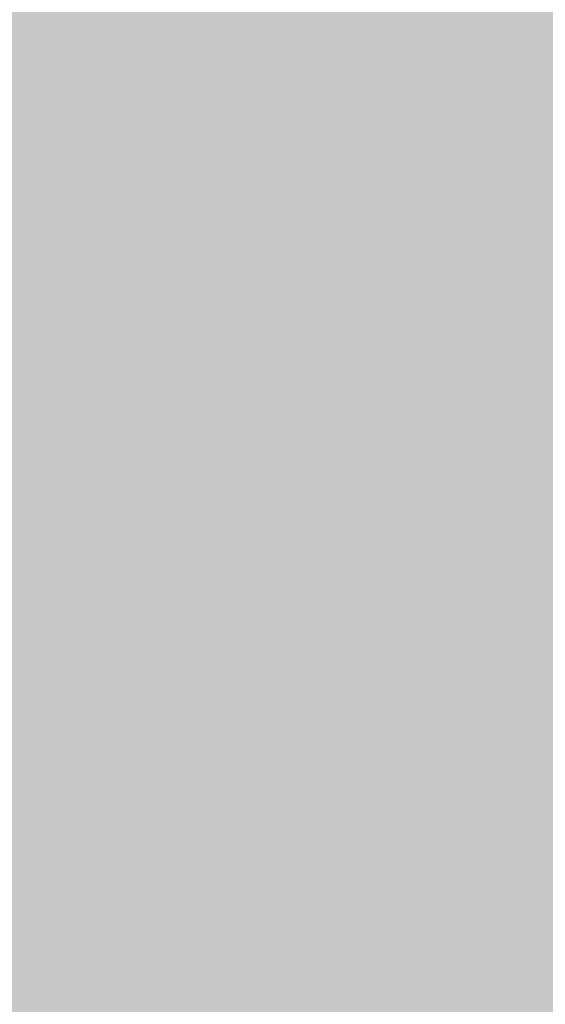
# Model space of a CAD drawing. Units: millimetres. Extents: x -22994 to 29398, y -19990 to 20176.
# Tile 61 of 135: x 225.441 to 227.437, y 79.586 to 83.328. Entities that reach past the tile are written whole.
import ezdxf
from ezdxf import colors
from ezdxf.entities.mleader import LeaderData, LeaderLine
from ezdxf.math import Vec2, Vec3

# ---------------------------------------------------------------- set-up
doc = ezdxf.new("R2010")
doc.units = ezdxf.units.MM
doc.header["$MEASUREMENT"] = 0
doc.layers.add('M-ANNO-TEXT', color=7, linetype='Continuous', lineweight=25)
doc.layers.add('M-DIMS', color=2, linetype='Continuous', lineweight=18)
doc.styles.get("Standard").update_dxf_attribs({"font": 'arial.ttf'})
doc.dimstyles.get("Standard").update_dxf_attribs({"dimtxt": 0.18, "dimasz": 10000, "dimexe": 0.18, "dimexo": 0.0625, "dimgap": 0.09, "dimtad": 0, "dimtih": 1, "dimtoh": 1, "dimdec": 0, "dimzin": 0, "dimdsep": 46, "dimtxsty": 'Standard', "dimcen": 0.09, "dimadec": 0, "dimazin": 0, "dimtfac": 1, "dimtdec": 0, "dimtofl": 0, "dimtmove": 0, "dimatfit": 3, "dimfxl": 1, "dimtolj": 1, "dimtzin": 0, "dimlwd": 30, "dimarcsym": 0})

# ---------------------------------------------------------------- blocks, each defined once
blk = doc.blocks.new('*D2')
at = {"layer": 'Defpoints', "color": 0, "transparency": 16777216}
for p in [(6.6773, 10.2713), (290.852, 10.2713), (290.852, -5.0787)]:
    blk.add_point(p, dxfattribs=at)
at = {"layer": 'M-DIMS', "color": 0, "lineweight": -2, "transparency": 16777216}
for p, q in [((6.6773, 10.2088), (6.6773, -5.2587)), ((290.852, 10.2088), (290.852, -5.2587))]:
    blk.add_line(p, q, dxfattribs=at)
at = {"layer": 'M-DIMS', "color": 0, "lineweight": 30, "transparency": 16777216}
for p, q in [((-9993.3227, -5.0787), (-19993.3227, -5.0787)), ((10290.852, -5.0787), (20290.852, -5.0787))]:
    blk.add_line(p, q, dxfattribs=at)
at = {"layer": 'M-DIMS', "color": 0, "transparency": 16777216}
for points in [[(-9993.3227, 1661.5879), (-9993.3227, -1671.7454), (6.6773, -5.0787)], [(10290.852, 1661.5879), (10290.852, -1671.7454), (290.852, -5.0787)]]:
    blk.add_solid(points, dxfattribs=at)
at = {"layer": 'M-DIMS', "color": 0, "transparency": 16777216, "insert": (148.7647, -5.0787), "char_height": 0.18, "attachment_point": 5}
blk.add_mtext('\\A1;284.2', dxfattribs=at)
blk = doc.blocks.new('*D3')
at = {"layer": 'Defpoints', "color": 0, "transparency": 16777216}
for p in [(110.2647, 204.1654), (110.2647, 176.3662), (95.8327, 127.967)]:
    blk.add_point(p, dxfattribs=at)
at = {"layer": 'M-DIMS', "color": 0, "lineweight": -2, "transparency": 16777216}
for p, q in [((95.8327, 128.0295), (95.8327, 204.3454)), ((110.2647, 176.4287), (110.2647, 204.3454))]:
    blk.add_line(p, q, dxfattribs=at)
at = {"layer": 'M-DIMS', "color": 0, "lineweight": 30, "transparency": 16777216}
for p, q in [((-9904.1673, 204.1654), (-19904.1673, 204.1654)), ((10110.2647, 204.1654), (20110.2647, 204.1654))]:
    blk.add_line(p, q, dxfattribs=at)
at = {"layer": 'M-DIMS', "color": 0, "transparency": 16777216}
for points in [[(-9904.1673, 1870.8321), (-9904.1673, -1462.5013), (95.8327, 204.1654)], [(10110.2647, 1870.8321), (10110.2647, -1462.5013), (110.2647, 204.1654)]]:
    blk.add_solid(points, dxfattribs=at)
at = {"layer": 'M-DIMS', "color": 0, "transparency": 16777216, "insert": (103.0487, 204.1654), "char_height": 0.18, "attachment_point": 5}
blk.add_mtext('\\A1;14.432', dxfattribs=at)
blk = doc.blocks.new('*D4')
at = {"layer": 'Defpoints', "color": 0, "transparency": 16777216}
for p in [(116.2647, 204.1654), (110.2647, 176.3662), (116.2647, 176.3662)]:
    blk.add_point(p, dxfattribs=at)
at = {"layer": 'M-DIMS', "color": 0, "lineweight": -2, "transparency": 16777216}
for p, q in [((110.2647, 176.4287), (110.2647, 204.3454)), ((116.2647, 176.4287), (116.2647, 204.3454))]:
    blk.add_line(p, q, dxfattribs=at)
at = {"layer": 'M-DIMS', "color": 0, "lineweight": 30, "transparency": 16777216}
for p, q in [((-9889.7353, 204.1654), (-19889.7353, 204.1654)), ((10116.2647, 204.1654), (20116.2647, 204.1654))]:
    blk.add_line(p, q, dxfattribs=at)
at = {"layer": 'M-DIMS', "color": 0, "transparency": 16777216}
for points in [[(-9889.7353, 1870.8321), (-9889.7353, -1462.5013), (110.2647, 204.1654)], [(10116.2647, 1870.8321), (10116.2647, -1462.5013), (116.2647, 204.1654)]]:
    blk.add_solid(points, dxfattribs=at)
at = {"layer": 'M-DIMS', "color": 0, "transparency": 16777216, "insert": (113.2647, 204.1654), "char_height": 0.18, "attachment_point": 5}
blk.add_mtext('\\A1;6', dxfattribs=at)
blk = doc.blocks.new('*D5')
at = {"layer": 'Defpoints', "color": 0, "transparency": 16777216}
for p in [(181.2647, 204.1654), (116.2647, 176.3662), (181.2647, 176.3662)]:
    blk.add_point(p, dxfattribs=at)
at = {"layer": 'M-DIMS', "color": 0, "lineweight": -2, "transparency": 16777216}
for p, q in [((116.2647, 176.4287), (116.2647, 204.3454)), ((181.2647, 176.4287), (181.2647, 204.3454))]:
    blk.add_line(p, q, dxfattribs=at)
at = {"layer": 'M-DIMS', "color": 0, "lineweight": 30, "transparency": 16777216}
for p, q in [((-9883.7353, 204.1654), (-19883.7353, 204.1654)), ((10181.2647, 204.1654), (20181.2647, 204.1654))]:
    blk.add_line(p, q, dxfattribs=at)
at = {"layer": 'M-DIMS', "color": 0, "transparency": 16777216}
for points in [[(-9883.7353, 1870.8321), (-9883.7353, -1462.5013), (116.2647, 204.1654)], [(10181.2647, 1870.8321), (10181.2647, -1462.5013), (181.2647, 204.1654)]]:
    blk.add_solid(points, dxfattribs=at)
at = {"layer": 'M-DIMS', "color": 0, "transparency": 16777216, "insert": (148.7647, 204.1654), "char_height": 0.18, "attachment_point": 5}
blk.add_mtext('\\A1;65', dxfattribs=at)
blk = doc.blocks.new('*D6')
at = {"layer": 'Defpoints', "color": 0, "transparency": 16777216}
for p in [(187.2647, 204.1654), (181.2647, 176.3662), (187.2647, 176.3662)]:
    blk.add_point(p, dxfattribs=at)
at = {"layer": 'M-DIMS', "color": 0, "lineweight": -2, "transparency": 16777216}
for p, q in [((181.2647, 176.4287), (181.2647, 204.3454)), ((187.2647, 176.4287), (187.2647, 204.3454))]:
    blk.add_line(p, q, dxfattribs=at)
at = {"layer": 'M-DIMS', "color": 0, "lineweight": 30, "transparency": 16777216}
for p, q in [((-9818.7353, 204.1654), (-19818.7353, 204.1654)), ((10187.2647, 204.1654), (20187.2647, 204.1654))]:
    blk.add_line(p, q, dxfattribs=at)
at = {"layer": 'M-DIMS', "color": 0, "transparency": 16777216}
for points in [[(-9818.7353, 1870.8321), (-9818.7353, -1462.5013), (181.2647, 204.1654)], [(10187.2647, 1870.8321), (10187.2647, -1462.5013), (187.2647, 204.1654)]]:
    blk.add_solid(points, dxfattribs=at)
at = {"layer": 'M-DIMS', "color": 0, "transparency": 16777216, "insert": (184.2647, 204.1654), "char_height": 0.18, "attachment_point": 5}
blk.add_mtext('\\A1;6', dxfattribs=at)
blk = doc.blocks.new('*D7')
at = {"layer": 'Defpoints', "color": 0, "transparency": 16777216}
for p in [(201.6967, 204.1654), (187.2647, 176.3662), (201.6967, 127.967)]:
    blk.add_point(p, dxfattribs=at)
at = {"layer": 'M-DIMS', "color": 0, "lineweight": -2, "transparency": 16777216}
for p, q in [((187.2647, 176.4287), (187.2647, 204.3454)), ((201.6967, 128.0295), (201.6967, 204.3454))]:
    blk.add_line(p, q, dxfattribs=at)
at = {"layer": 'M-DIMS', "color": 0, "lineweight": 30, "transparency": 16777216}
for p, q in [((-9812.7353, 204.1654), (-19812.7353, 204.1654)), ((10201.6967, 204.1654), (20201.6967, 204.1654))]:
    blk.add_line(p, q, dxfattribs=at)
at = {"layer": 'M-DIMS', "color": 0, "transparency": 16777216}
for points in [[(-9812.7353, 1870.8321), (-9812.7353, -1462.5013), (187.2647, 204.1654)], [(10201.6967, 1870.8321), (10201.6967, -1462.5013), (201.6967, 204.1654)]]:
    blk.add_solid(points, dxfattribs=at)
at = {"layer": 'M-DIMS', "color": 0, "transparency": 16777216, "insert": (194.4807, 204.1654), "char_height": 0.18, "attachment_point": 5}
blk.add_mtext('\\A1;14.432', dxfattribs=at)
blk = doc.blocks.new('*D8')
at = {"layer": 'Defpoints', "color": 0, "transparency": 16777216}
for p in [(227.6485, 204.1654), (227.6485, 146.7296), (201.6967, 127.967)]:
    blk.add_point(p, dxfattribs=at)
at = {"layer": 'M-DIMS', "color": 0, "lineweight": -2, "transparency": 16777216}
for p, q in [((201.6967, 128.0295), (201.6967, 204.3454)), ((227.6485, 146.7921), (227.6485, 204.3454))]:
    blk.add_line(p, q, dxfattribs=at)
at = {"layer": 'M-DIMS', "color": 0, "lineweight": 30, "transparency": 16777216}
for p, q in [((-9798.3033, 204.1654), (-19798.3033, 204.1654)), ((10227.6485, 204.1654), (20227.6485, 204.1654))]:
    blk.add_line(p, q, dxfattribs=at)
at = {"layer": 'M-DIMS', "color": 0, "transparency": 16777216}
for points in [[(-9798.3033, 1870.8321), (-9798.3033, -1462.5013), (201.6967, 204.1654)], [(10227.6485, 1870.8321), (10227.6485, -1462.5013), (227.6485, 204.1654)]]:
    blk.add_solid(points, dxfattribs=at)
at = {"layer": 'M-DIMS', "color": 0, "transparency": 16777216, "insert": (214.6726, 204.1654), "char_height": 0.18, "attachment_point": 5}
blk.add_mtext('\\A1;25.95', dxfattribs=at)
blk = doc.blocks.new('*D9')
at = {"layer": 'Defpoints', "color": 0, "transparency": 16777216}
for p in [(187.2647, 176.3662), (306.202, 176.3662), (290.852, 10.2713)]:
    blk.add_point(p, dxfattribs=at)
at = {"layer": 'M-DIMS', "color": 0, "lineweight": 30, "transparency": 16777216}
for p, q in [((306.202, 10176.3662), (306.202, 20176.3662)), ((306.202, -9989.7287), (306.202, -19989.7287))]:
    blk.add_line(p, q, dxfattribs=at)
at = {"layer": 'M-DIMS', "color": 0, "lineweight": -2, "transparency": 16777216}
for p, q in [((187.3272, 176.3662), (306.382, 176.3662)), ((290.9145, 10.2713), (306.382, 10.2713))]:
    blk.add_line(p, q, dxfattribs=at)
at = {"layer": 'M-DIMS', "color": 0, "transparency": 16777216}
for points in [[(-1360.4646, 10176.3662), (1972.8687, 10176.3662), (306.202, 176.3662)], [(-1360.4646, -9989.7287), (1972.8687, -9989.7287), (306.202, 10.2713)]]:
    blk.add_solid(points, dxfattribs=at)
at = {"layer": 'M-DIMS', "color": 0, "transparency": 16777216, "insert": (306.202, 93.3187), "char_height": 0.18, "attachment_point": 5}
blk.add_mtext('\\A1;166.1', dxfattribs=at)
blk = doc.blocks.new('*D10')
at = {"layer": 'Defpoints', "color": 0, "transparency": 16777216}
for p in [(125.6498, 136.0713), (133.3459, 136.0713), (133.3459, -5.0787)]:
    blk.add_point(p, dxfattribs=at)
at = {"layer": 'M-DIMS', "color": 0, "lineweight": -2, "transparency": 16777216}
for p, q in [((125.6498, 136.0088), (125.6498, -5.2587)), ((133.3459, 136.0088), (133.3459, -5.2587))]:
    blk.add_line(p, q, dxfattribs=at)
at = {"layer": 'M-DIMS', "color": 0, "lineweight": 30, "transparency": 16777216}
for p, q in [((-9874.3502, -5.0787), (-19874.3502, -5.0787)), ((10133.3459, -5.0787), (20133.3459, -5.0787))]:
    blk.add_line(p, q, dxfattribs=at)
at = {"layer": 'M-DIMS', "color": 0, "transparency": 16777216}
for points in [[(-9874.3502, 1661.5879), (-9874.3502, -1671.7454), (125.6498, -5.0787)], [(10133.3459, 1661.5879), (10133.3459, -1671.7454), (133.3459, -5.0787)]]:
    blk.add_solid(points, dxfattribs=at)
at = {"layer": 'M-DIMS', "color": 0, "transparency": 16777216, "insert": (129.4978, -5.0787), "char_height": 0.18, "attachment_point": 5}
blk.add_mtext('\\A1;7.696', dxfattribs=at)
blk = doc.blocks.new('*D11')
at = {"layer": 'Defpoints', "color": 0, "transparency": 16777216}
for p in [(133.3459, 136.0713), (135.6498, 136.0713), (135.6498, -5.0787)]:
    blk.add_point(p, dxfattribs=at)
at = {"layer": 'M-DIMS', "color": 0, "lineweight": -2, "transparency": 16777216}
for p, q in [((133.3459, 136.0088), (133.3459, -5.2587)), ((135.6498, 136.0088), (135.6498, -5.2587))]:
    blk.add_line(p, q, dxfattribs=at)
at = {"layer": 'M-DIMS', "color": 0, "lineweight": 30, "transparency": 16777216}
for p, q in [((-9866.6541, -5.0787), (-19866.6541, -5.0787)), ((10135.6498, -5.0787), (20135.6498, -5.0787))]:
    blk.add_line(p, q, dxfattribs=at)
at = {"layer": 'M-DIMS', "color": 0, "transparency": 16777216}
for points in [[(-9866.6541, 1661.5879), (-9866.6541, -1671.7454), (133.3459, -5.0787)], [(10135.6498, 1661.5879), (10135.6498, -1671.7454), (135.6498, -5.0787)]]:
    blk.add_solid(points, dxfattribs=at)
at = {"layer": 'M-DIMS', "color": 0, "transparency": 16777216, "insert": (134.4978, -5.0787), "char_height": 0.18, "attachment_point": 5}
blk.add_mtext('\\A1;2.304', dxfattribs=at)
blk = doc.blocks.new('*D12')
at = {"layer": 'Defpoints', "color": 0, "transparency": 16777216}
for p in [(135.6498, 136.0713), (145.6498, 136.0713), (145.6498, -5.0787)]:
    blk.add_point(p, dxfattribs=at)
at = {"layer": 'M-DIMS', "color": 0, "lineweight": -2, "transparency": 16777216}
for p, q in [((135.6498, 136.0088), (135.6498, -5.2587)), ((145.6498, 136.0088), (145.6498, -5.2587))]:
    blk.add_line(p, q, dxfattribs=at)
at = {"layer": 'M-DIMS', "color": 0, "lineweight": 30, "transparency": 16777216}
for p, q in [((-9864.3502, -5.0787), (-19864.3502, -5.0787)), ((10145.6498, -5.0787), (20145.6498, -5.0787))]:
    blk.add_line(p, q, dxfattribs=at)
at = {"layer": 'M-DIMS', "color": 0, "transparency": 16777216}
for points in [[(-9864.3502, 1661.5879), (-9864.3502, -1671.7454), (135.6498, -5.0787)], [(10145.6498, 1661.5879), (10145.6498, -1671.7454), (145.6498, -5.0787)]]:
    blk.add_solid(points, dxfattribs=at)
at = {"layer": 'M-DIMS', "color": 0, "transparency": 16777216, "insert": (140.6498, -5.0787), "char_height": 0.18, "attachment_point": 5}
blk.add_mtext('\\A1;10', dxfattribs=at)
blk = doc.blocks.new('*D13')
at = {"layer": 'Defpoints', "color": 0, "transparency": 16777216}
for p in [(145.6498, 136.0713), (155.6498, 136.0713), (155.6498, -5.0787)]:
    blk.add_point(p, dxfattribs=at)
at = {"layer": 'M-DIMS', "color": 0, "lineweight": -2, "transparency": 16777216}
for p, q in [((145.6498, 136.0088), (145.6498, -5.2587)), ((155.6498, 136.0088), (155.6498, -5.2587))]:
    blk.add_line(p, q, dxfattribs=at)
at = {"layer": 'M-DIMS', "color": 0, "lineweight": 30, "transparency": 16777216}
for p, q in [((-9854.3502, -5.0787), (-19854.3502, -5.0787)), ((10155.6498, -5.0787), (20155.6498, -5.0787))]:
    blk.add_line(p, q, dxfattribs=at)
at = {"layer": 'M-DIMS', "color": 0, "transparency": 16777216}
for points in [[(-9854.3502, 1661.5879), (-9854.3502, -1671.7454), (145.6498, -5.0787)], [(10155.6498, 1661.5879), (10155.6498, -1671.7454), (155.6498, -5.0787)]]:
    blk.add_solid(points, dxfattribs=at)
at = {"layer": 'M-DIMS', "color": 0, "transparency": 16777216, "insert": (150.6498, -5.0787), "char_height": 0.18, "attachment_point": 5}
blk.add_mtext('\\A1;10', dxfattribs=at)
blk = doc.blocks.new('*D14')
at = {"layer": 'Defpoints', "color": 0, "transparency": 16777216}
for p in [(155.6498, 136.0713), (165.6498, 136.0713), (165.6498, -5.0787)]:
    blk.add_point(p, dxfattribs=at)
at = {"layer": 'M-DIMS', "color": 0, "lineweight": -2, "transparency": 16777216}
for p, q in [((155.6498, 136.0088), (155.6498, -5.2587)), ((165.6498, 136.0088), (165.6498, -5.2587))]:
    blk.add_line(p, q, dxfattribs=at)
at = {"layer": 'M-DIMS', "color": 0, "lineweight": 30, "transparency": 16777216}
for p, q in [((-9844.3502, -5.0787), (-19844.3502, -5.0787)), ((10165.6498, -5.0787), (20165.6498, -5.0787))]:
    blk.add_line(p, q, dxfattribs=at)
at = {"layer": 'M-DIMS', "color": 0, "transparency": 16777216}
for points in [[(-9844.3502, 1661.5879), (-9844.3502, -1671.7454), (155.6498, -5.0787)], [(10165.6498, 1661.5879), (10165.6498, -1671.7454), (165.6498, -5.0787)]]:
    blk.add_solid(points, dxfattribs=at)
at = {"layer": 'M-DIMS', "color": 0, "transparency": 16777216, "insert": (160.6498, -5.0787), "char_height": 0.18, "attachment_point": 5}
blk.add_mtext('\\A1;10', dxfattribs=at)
blk = doc.blocks.new('*D15')
at = {"layer": 'Defpoints', "color": 0, "transparency": 16777216}
for p in [(173.3459, 154.788), (173.3459, 136.0713), (306.202, 136.0713)]:
    blk.add_point(p, dxfattribs=at)
at = {"layer": 'M-DIMS', "color": 0, "lineweight": 30, "transparency": 16777216}
for p, q in [((306.202, 10154.788), (306.202, 20154.788)), ((306.202, -9863.9287), (306.202, -19863.9287))]:
    blk.add_line(p, q, dxfattribs=at)
at = {"layer": 'M-DIMS', "color": 0, "lineweight": -2, "transparency": 16777216}
for p, q in [((173.4084, 154.788), (306.382, 154.788)), ((173.4084, 136.0713), (306.382, 136.0713))]:
    blk.add_line(p, q, dxfattribs=at)
at = {"layer": 'M-DIMS', "color": 0, "transparency": 16777216}
for points in [[(-1360.4646, 10154.788), (1972.8687, 10154.788), (306.202, 154.788)], [(-1360.4646, -9863.9287), (1972.8687, -9863.9287), (306.202, 136.0713)]]:
    blk.add_solid(points, dxfattribs=at)
at = {"layer": 'M-DIMS', "color": 0, "transparency": 16777216, "insert": (306.202, 145.4297), "char_height": 0.18, "attachment_point": 5}
blk.add_mtext('\\A1;18.717', dxfattribs=at)
blk = doc.blocks.new('*D16')
at = {"layer": 'Defpoints', "color": 0, "transparency": 16777216}
for p in [(120.1702, 204.1654), (110.4658, 48.0349), (120.1702, 48.0349)]:
    blk.add_point(p, dxfattribs=at)
at = {"layer": 'M-DIMS', "color": 0, "lineweight": -2, "transparency": 16777216}
for p, q in [((110.4658, 48.0974), (110.4658, 204.3454)), ((120.1702, 48.0974), (120.1702, 204.3454))]:
    blk.add_line(p, q, dxfattribs=at)
at = {"layer": 'M-DIMS', "color": 0, "lineweight": 30, "transparency": 16777216}
for p, q in [((-9889.5342, 204.1654), (-19889.5342, 204.1654)), ((10120.1702, 204.1654), (20120.1702, 204.1654))]:
    blk.add_line(p, q, dxfattribs=at)
at = {"layer": 'M-DIMS', "color": 0, "transparency": 16777216}
for points in [[(-9889.5342, 1870.8321), (-9889.5342, -1462.5013), (110.4658, 204.1654)], [(10120.1702, 1870.8321), (10120.1702, -1462.5013), (120.1702, 204.1654)]]:
    blk.add_solid(points, dxfattribs=at)
at = {"layer": 'M-DIMS', "color": 0, "transparency": 16777216, "insert": (115.318, 204.1654), "char_height": 0.18, "attachment_point": 5}
blk.add_mtext('\\A1;9.704', dxfattribs=at)
blk = doc.blocks.new('*D17')
at = {"layer": 'Defpoints', "color": 0, "transparency": 16777216}
for p in [(126.1702, 204.1654), (120.1702, 48.0349), (126.1702, 48.0349)]:
    blk.add_point(p, dxfattribs=at)
at = {"layer": 'M-DIMS', "color": 0, "lineweight": -2, "transparency": 16777216}
for p, q in [((120.1702, 48.0974), (120.1702, 204.3454)), ((126.1702, 48.0974), (126.1702, 204.3454))]:
    blk.add_line(p, q, dxfattribs=at)
at = {"layer": 'M-DIMS', "color": 0, "lineweight": 30, "transparency": 16777216}
for p, q in [((-9879.8298, 204.1654), (-19879.8298, 204.1654)), ((10126.1702, 204.1654), (20126.1702, 204.1654))]:
    blk.add_line(p, q, dxfattribs=at)
at = {"layer": 'M-DIMS', "color": 0, "transparency": 16777216}
for points in [[(-9879.8298, 1870.8321), (-9879.8298, -1462.5013), (120.1702, 204.1654)], [(10126.1702, 1870.8321), (10126.1702, -1462.5013), (126.1702, 204.1654)]]:
    blk.add_solid(points, dxfattribs=at)
at = {"layer": 'M-DIMS', "color": 0, "transparency": 16777216, "insert": (123.1702, 204.1654), "char_height": 0.18, "attachment_point": 5}
blk.add_mtext('\\A1;6', dxfattribs=at)
blk = doc.blocks.new('*D18')
at = {"layer": 'Defpoints', "color": 0, "transparency": 16777216}
for p in [(132.1702, 204.1654), (126.1702, 48.0349), (132.1702, 48.0349)]:
    blk.add_point(p, dxfattribs=at)
at = {"layer": 'M-DIMS', "color": 0, "lineweight": -2, "transparency": 16777216}
for p, q in [((126.1702, 48.0974), (126.1702, 204.3454)), ((132.1702, 48.0974), (132.1702, 204.3454))]:
    blk.add_line(p, q, dxfattribs=at)
at = {"layer": 'M-DIMS', "color": 0, "lineweight": 30, "transparency": 16777216}
for p, q in [((-9873.8298, 204.1654), (-19873.8298, 204.1654)), ((10132.1702, 204.1654), (20132.1702, 204.1654))]:
    blk.add_line(p, q, dxfattribs=at)
at = {"layer": 'M-DIMS', "color": 0, "transparency": 16777216}
for points in [[(-9873.8298, 1870.8321), (-9873.8298, -1462.5013), (126.1702, 204.1654)], [(10132.1702, 1870.8321), (10132.1702, -1462.5013), (132.1702, 204.1654)]]:
    blk.add_solid(points, dxfattribs=at)
at = {"layer": 'M-DIMS', "color": 0, "transparency": 16777216, "insert": (129.1702, 204.1654), "char_height": 0.18, "attachment_point": 5}
blk.add_mtext('\\A1;6', dxfattribs=at)
blk = doc.blocks.new('*D19')
at = {"layer": 'Defpoints', "color": 0, "transparency": 16777216}
for p in [(138.1702, 204.1654), (132.1702, 48.0349), (138.1702, 48.0349)]:
    blk.add_point(p, dxfattribs=at)
at = {"layer": 'M-DIMS', "color": 0, "lineweight": -2, "transparency": 16777216}
for p, q in [((132.1702, 48.0974), (132.1702, 204.3454)), ((138.1702, 48.0974), (138.1702, 204.3454))]:
    blk.add_line(p, q, dxfattribs=at)
at = {"layer": 'M-DIMS', "color": 0, "lineweight": 30, "transparency": 16777216}
for p, q in [((-9867.8298, 204.1654), (-19867.8298, 204.1654)), ((10138.1702, 204.1654), (20138.1702, 204.1654))]:
    blk.add_line(p, q, dxfattribs=at)
at = {"layer": 'M-DIMS', "color": 0, "transparency": 16777216}
for points in [[(-9867.8298, 1870.8321), (-9867.8298, -1462.5013), (132.1702, 204.1654)], [(10138.1702, 1870.8321), (10138.1702, -1462.5013), (138.1702, 204.1654)]]:
    blk.add_solid(points, dxfattribs=at)
at = {"layer": 'M-DIMS', "color": 0, "transparency": 16777216, "insert": (135.1702, 204.1654), "char_height": 0.18, "attachment_point": 5}
blk.add_mtext('\\A1;6', dxfattribs=at)
blk = doc.blocks.new('*D20')
at = {"layer": 'Defpoints', "color": 0, "transparency": 16777216}
for p in [(144.1702, 204.1654), (138.1702, 48.0349), (144.1702, 48.0349)]:
    blk.add_point(p, dxfattribs=at)
at = {"layer": 'M-DIMS', "color": 0, "lineweight": -2, "transparency": 16777216}
for p, q in [((138.1702, 48.0974), (138.1702, 204.3454)), ((144.1702, 48.0974), (144.1702, 204.3454))]:
    blk.add_line(p, q, dxfattribs=at)
at = {"layer": 'M-DIMS', "color": 0, "lineweight": 30, "transparency": 16777216}
for p, q in [((-9861.8298, 204.1654), (-19861.8298, 204.1654)), ((10144.1702, 204.1654), (20144.1702, 204.1654))]:
    blk.add_line(p, q, dxfattribs=at)
at = {"layer": 'M-DIMS', "color": 0, "transparency": 16777216}
for points in [[(-9861.8298, 1870.8321), (-9861.8298, -1462.5013), (138.1702, 204.1654)], [(10144.1702, 1870.8321), (10144.1702, -1462.5013), (144.1702, 204.1654)]]:
    blk.add_solid(points, dxfattribs=at)
at = {"layer": 'M-DIMS', "color": 0, "transparency": 16777216, "insert": (141.1702, 204.1654), "char_height": 0.18, "attachment_point": 5}
blk.add_mtext('\\A1;6', dxfattribs=at)
blk = doc.blocks.new('*D21')
at = {"layer": 'Defpoints', "color": 0, "transparency": 16777216}
for p in [(149.1157, 204.1654), (144.1702, 48.0349), (149.1157, 48.0349)]:
    blk.add_point(p, dxfattribs=at)
at = {"layer": 'M-DIMS', "color": 0, "lineweight": -2, "transparency": 16777216}
for p, q in [((144.1702, 48.0974), (144.1702, 204.3454)), ((149.1157, 48.0974), (149.1157, 204.3454))]:
    blk.add_line(p, q, dxfattribs=at)
at = {"layer": 'M-DIMS', "color": 0, "lineweight": 30, "transparency": 16777216}
for p, q in [((-9855.8298, 204.1654), (-19855.8298, 204.1654)), ((10149.1157, 204.1654), (20149.1157, 204.1654))]:
    blk.add_line(p, q, dxfattribs=at)
at = {"layer": 'M-DIMS', "color": 0, "transparency": 16777216}
for points in [[(-9855.8298, 1870.8321), (-9855.8298, -1462.5013), (144.1702, 204.1654)], [(10149.1157, 1870.8321), (10149.1157, -1462.5013), (149.1157, 204.1654)]]:
    blk.add_solid(points, dxfattribs=at)
at = {"layer": 'M-DIMS', "color": 0, "transparency": 16777216, "insert": (146.6429, 204.1654), "char_height": 0.18, "attachment_point": 5}
blk.add_mtext('\\A1;4.945', dxfattribs=at)
blk = doc.blocks.new('*D22')
at = {"layer": 'Defpoints', "color": 0, "transparency": 16777216}
for p in [(149.1157, 30.9895), (155.1157, 30.9895), (155.1157, -5.0787)]:
    blk.add_point(p, dxfattribs=at)
at = {"layer": 'M-DIMS', "color": 0, "lineweight": -2, "transparency": 16777216}
for p, q in [((149.1157, 30.927), (149.1157, -5.2587)), ((155.1157, 30.927), (155.1157, -5.2587))]:
    blk.add_line(p, q, dxfattribs=at)
at = {"layer": 'M-DIMS', "color": 0, "lineweight": 30, "transparency": 16777216}
for p, q in [((-9850.8843, -5.0787), (-19850.8843, -5.0787)), ((10155.1157, -5.0787), (20155.1157, -5.0787))]:
    blk.add_line(p, q, dxfattribs=at)
at = {"layer": 'M-DIMS', "color": 0, "transparency": 16777216}
for points in [[(-9850.8843, 1661.5879), (-9850.8843, -1671.7454), (149.1157, -5.0787)], [(10155.1157, 1661.5879), (10155.1157, -1671.7454), (155.1157, -5.0787)]]:
    blk.add_solid(points, dxfattribs=at)
at = {"layer": 'M-DIMS', "color": 0, "transparency": 16777216, "insert": (152.1157, -5.0787), "char_height": 0.18, "attachment_point": 5}
blk.add_mtext('\\A1;6', dxfattribs=at)
blk = doc.blocks.new('*D23')
at = {"layer": 'Defpoints', "color": 0, "transparency": 16777216}
for p in [(155.1157, 30.9895), (161.1157, 30.9895), (161.1157, -5.0787)]:
    blk.add_point(p, dxfattribs=at)
at = {"layer": 'M-DIMS', "color": 0, "lineweight": -2, "transparency": 16777216}
for p, q in [((155.1157, 30.927), (155.1157, -5.2587)), ((161.1157, 30.927), (161.1157, -5.2587))]:
    blk.add_line(p, q, dxfattribs=at)
at = {"layer": 'M-DIMS', "color": 0, "lineweight": 30, "transparency": 16777216}
for p, q in [((-9844.8843, -5.0787), (-19844.8843, -5.0787)), ((10161.1157, -5.0787), (20161.1157, -5.0787))]:
    blk.add_line(p, q, dxfattribs=at)
at = {"layer": 'M-DIMS', "color": 0, "transparency": 16777216}
for points in [[(-9844.8843, 1661.5879), (-9844.8843, -1671.7454), (155.1157, -5.0787)], [(10161.1157, 1661.5879), (10161.1157, -1671.7454), (161.1157, -5.0787)]]:
    blk.add_solid(points, dxfattribs=at)
at = {"layer": 'M-DIMS', "color": 0, "transparency": 16777216, "insert": (158.1157, -5.0787), "char_height": 0.18, "attachment_point": 5}
blk.add_mtext('\\A1;6', dxfattribs=at)
blk = doc.blocks.new('*D24')
at = {"layer": 'Defpoints', "color": 0, "transparency": 16777216}
for p in [(161.1157, 30.9895), (166.4387, 30.9895), (166.4387, -5.0787)]:
    blk.add_point(p, dxfattribs=at)
at = {"layer": 'M-DIMS', "color": 0, "lineweight": -2, "transparency": 16777216}
for p, q in [((161.1157, 30.927), (161.1157, -5.2587)), ((166.4387, 30.927), (166.4387, -5.2587))]:
    blk.add_line(p, q, dxfattribs=at)
at = {"layer": 'M-DIMS', "color": 0, "lineweight": 30, "transparency": 16777216}
for p, q in [((-9838.8843, -5.0787), (-19838.8843, -5.0787)), ((10166.4387, -5.0787), (20166.4387, -5.0787))]:
    blk.add_line(p, q, dxfattribs=at)
at = {"layer": 'M-DIMS', "color": 0, "transparency": 16777216}
for points in [[(-9838.8843, 1661.5879), (-9838.8843, -1671.7454), (161.1157, -5.0787)], [(10166.4387, 1661.5879), (10166.4387, -1671.7454), (166.4387, -5.0787)]]:
    blk.add_solid(points, dxfattribs=at)
at = {"layer": 'M-DIMS', "color": 0, "transparency": 16777216, "insert": (163.7772, -5.0787), "char_height": 0.18, "attachment_point": 5}
blk.add_mtext('\\A1;5.323', dxfattribs=at)
blk = doc.blocks.new('*D25')
at = {"layer": 'Defpoints', "color": 0, "transparency": 16777216}
for p in [(166.4387, 30.9895), (172.4387, 30.9895), (172.4387, -5.0787)]:
    blk.add_point(p, dxfattribs=at)
at = {"layer": 'M-DIMS', "color": 0, "lineweight": -2, "transparency": 16777216}
for p, q in [((166.4387, 30.927), (166.4387, -5.2587)), ((172.4387, 30.927), (172.4387, -5.2587))]:
    blk.add_line(p, q, dxfattribs=at)
at = {"layer": 'M-DIMS', "color": 0, "lineweight": 30, "transparency": 16777216}
for p, q in [((-9833.5613, -5.0787), (-19833.5613, -5.0787)), ((10172.4387, -5.0787), (20172.4387, -5.0787))]:
    blk.add_line(p, q, dxfattribs=at)
at = {"layer": 'M-DIMS', "color": 0, "transparency": 16777216}
for points in [[(-9833.5613, 1661.5879), (-9833.5613, -1671.7454), (166.4387, -5.0787)], [(10172.4387, 1661.5879), (10172.4387, -1671.7454), (172.4387, -5.0787)]]:
    blk.add_solid(points, dxfattribs=at)
at = {"layer": 'M-DIMS', "color": 0, "transparency": 16777216, "insert": (169.4387, -5.0787), "char_height": 0.18, "attachment_point": 5}
blk.add_mtext('\\A1;6', dxfattribs=at)
blk = doc.blocks.new('*D26')
at = {"layer": 'Defpoints', "color": 0, "transparency": 16777216}
for p in [(172.4387, 30.9895), (178.4387, 30.9895), (178.4387, -5.0787)]:
    blk.add_point(p, dxfattribs=at)
at = {"layer": 'M-DIMS', "color": 0, "lineweight": -2, "transparency": 16777216}
for p, q in [((172.4387, 30.927), (172.4387, -5.2587)), ((178.4387, 30.927), (178.4387, -5.2587))]:
    blk.add_line(p, q, dxfattribs=at)
at = {"layer": 'M-DIMS', "color": 0, "lineweight": 30, "transparency": 16777216}
for p, q in [((-9827.5613, -5.0787), (-19827.5613, -5.0787)), ((10178.4387, -5.0787), (20178.4387, -5.0787))]:
    blk.add_line(p, q, dxfattribs=at)
at = {"layer": 'M-DIMS', "color": 0, "transparency": 16777216}
for points in [[(-9827.5613, 1661.5879), (-9827.5613, -1671.7454), (172.4387, -5.0787)], [(10178.4387, 1661.5879), (10178.4387, -1671.7454), (178.4387, -5.0787)]]:
    blk.add_solid(points, dxfattribs=at)
at = {"layer": 'M-DIMS', "color": 0, "transparency": 16777216, "insert": (175.4387, -5.0787), "char_height": 0.18, "attachment_point": 5}
blk.add_mtext('\\A1;6', dxfattribs=at)
blk = doc.blocks.new('*D27')
at = {"layer": 'Defpoints', "color": 0, "transparency": 16777216}
for p in [(178.4387, 30.9895), (188.1175, 30.9895), (188.1175, -5.0787)]:
    blk.add_point(p, dxfattribs=at)
at = {"layer": 'M-DIMS', "color": 0, "lineweight": -2, "transparency": 16777216}
for p, q in [((178.4387, 30.927), (178.4387, -5.2587)), ((188.1175, 30.927), (188.1175, -5.2587))]:
    blk.add_line(p, q, dxfattribs=at)
at = {"layer": 'M-DIMS', "color": 0, "lineweight": 30, "transparency": 16777216}
for p, q in [((-9821.5613, -5.0787), (-19821.5613, -5.0787)), ((10188.1175, -5.0787), (20188.1175, -5.0787))]:
    blk.add_line(p, q, dxfattribs=at)
at = {"layer": 'M-DIMS', "color": 0, "transparency": 16777216}
for points in [[(-9821.5613, 1661.5879), (-9821.5613, -1671.7454), (178.4387, -5.0787)], [(10188.1175, 1661.5879), (10188.1175, -1671.7454), (188.1175, -5.0787)]]:
    blk.add_solid(points, dxfattribs=at)
at = {"layer": 'M-DIMS', "color": 0, "transparency": 16777216, "insert": (183.2781, -5.0787), "char_height": 0.18, "attachment_point": 5}
blk.add_mtext('\\A1;9.679', dxfattribs=at)
blk = doc.blocks.new('*D28')
at = {"layer": 'Defpoints', "color": 0, "transparency": 16777216}
for p in [(188.1175, 48.0349), (306.202, 48.0349), (188.1175, 30.9895)]:
    blk.add_point(p, dxfattribs=at)
at = {"layer": 'M-DIMS', "color": 0, "lineweight": 30, "transparency": 16777216}
for p, q in [((306.202, 10048.0349), (306.202, 20048.0349)), ((306.202, -9969.0105), (306.202, -19969.0105))]:
    blk.add_line(p, q, dxfattribs=at)
at = {"layer": 'M-DIMS', "color": 0, "lineweight": -2, "transparency": 16777216}
for p, q in [((188.18, 48.0349), (306.382, 48.0349)), ((188.18, 30.9895), (306.382, 30.9895))]:
    blk.add_line(p, q, dxfattribs=at)
at = {"layer": 'M-DIMS', "color": 0, "transparency": 16777216}
for points in [[(-1360.4646, 10048.0349), (1972.8687, 10048.0349), (306.202, 48.0349)], [(-1360.4646, -9969.0105), (1972.8687, -9969.0105), (306.202, 30.9895)]]:
    blk.add_solid(points, dxfattribs=at)
at = {"layer": 'M-DIMS', "color": 0, "transparency": 16777216, "insert": (306.202, 39.5122), "char_height": 0.18, "attachment_point": 5}
blk.add_mtext('\\A1;17.045', dxfattribs=at)
blk = doc.blocks.new('*D29')
at = {"layer": 'Defpoints', "color": 0, "transparency": 16777216}
for p in [(36.8006, 80.045), (64.0296, 80.045)]:
    blk.add_point(p, dxfattribs=at)
at = {"layer": 'M-DIMS', "color": 0, "lineweight": -2, "transparency": 16777216}
for p, q in [((50.4151, 79.955), (50.4151, 80.135)), ((50.3251, 80.045), (50.5051, 80.045))]:
    blk.add_line(p, q, dxfattribs=at)
at = {"layer": 'M-DIMS', "color": 0, "lineweight": 30, "transparency": 16777216}
blk.add_line((20064.0296, 80.0303), (10064.0296, 80.0377), dxfattribs=at)
at = {"layer": 'M-DIMS', "color": 0, "transparency": 16777216}
blk.add_solid([(10064.0309, 1746.7043), (10064.0284, -1586.629), (64.0296, 80.045)], dxfattribs=at)
at = {"layer": 'M-DIMS', "color": 0, "transparency": 16777216, "insert": (20064.5213, 80.0303), "char_height": 0.18, "attachment_point": 5}
blk.add_mtext('\\A1;∅27.23', dxfattribs=at)
blk = doc.blocks.new('*D30')
at = {"layer": 'Defpoints', "color": 0, "transparency": 16777216}
for p in [(216.3148, 146.7291), (238.9821, 146.73)]:
    blk.add_point(p, dxfattribs=at)
at = {"layer": 'M-DIMS', "color": 0, "lineweight": 30, "transparency": 16777216}
blk.add_line((20238.9821, 147.4959), (10238.9821, 147.1129), dxfattribs=at)
at = {"layer": 'M-DIMS', "color": 0, "lineweight": -2, "transparency": 16777216}
for p, q in [((227.6485, 146.6396), (227.6485, 146.8196)), ((227.5585, 146.7296), (227.7385, 146.7296))]:
    blk.add_line(p, q, dxfattribs=at)
at = {"layer": 'M-DIMS', "color": 0, "transparency": 16777216}
blk.add_solid([(10238.9183, 1813.7796), (10239.0459, -1519.5537), (238.9821, 146.73)], dxfattribs=at)
at = {"layer": 'M-DIMS', "color": 0, "transparency": 16777216, "insert": (20239.5436, 147.4959), "char_height": 0.18, "attachment_point": 5}
blk.add_mtext('\\A1;∅22.667', dxfattribs=at)
blk = doc.blocks.new('*D31')
at = {"layer": 'Defpoints', "color": 0, "transparency": 16777216}
for p in [(223.1641, 146.7291), (232.1328, 146.73)]:
    blk.add_point(p, dxfattribs=at)
at = {"layer": 'M-DIMS', "color": 0, "lineweight": 30, "transparency": 16777216}
blk.add_line((20232.1327, 148.6656), (10232.1328, 147.6978), dxfattribs=at)
at = {"layer": 'M-DIMS', "color": 0, "lineweight": -2, "transparency": 16777216}
for p, q in [((227.6485, 146.6396), (227.6485, 146.8196)), ((227.5585, 146.7296), (227.7385, 146.7296))]:
    blk.add_line(p, q, dxfattribs=at)
at = {"layer": 'M-DIMS', "color": 0, "transparency": 16777216}
blk.add_solid([(10231.9715, 1814.3645), (10232.2941, -1518.9688), (232.1328, 146.73)], dxfattribs=at)
at = {"layer": 'M-DIMS', "color": 0, "transparency": 16777216, "insert": (20232.6245, 148.6656), "char_height": 0.18, "attachment_point": 5}
blk.add_mtext('\\A1;∅8.969', dxfattribs=at)
blk = doc.blocks.new('*D36')
at = {"layer": 'Defpoints', "color": 0, "transparency": 16777216}
for p in [(46.39, 31.3035), (46.3875, 26.5934)]:
    blk.add_point(p, dxfattribs=at)
at = {"layer": 'M-DIMS', "color": 0, "lineweight": 30, "transparency": 16777216}
for p, q in [((57.1499, 20031.3006), (51.77, 10031.302)), ((10057.1499, 20031.3006), (57.1499, 20031.3006))]:
    blk.add_line(p, q, dxfattribs=at)
at = {"layer": 'M-DIMS', "color": 0, "lineweight": -2, "transparency": 16777216}
for p, q in [((46.3887, 28.8585), (46.3887, 29.0385)), ((46.2987, 28.9485), (46.4787, 28.9485))]:
    blk.add_line(p, q, dxfattribs=at)
at = {"layer": 'M-DIMS', "color": 0, "transparency": 16777216}
blk.add_solid([(-1614.8965, 10032.1987), (1718.4364, 10030.4054), (46.39, 31.3035)], dxfattribs=at)
at = {"layer": 'M-DIMS', "color": 0, "transparency": 16777216, "insert": (10057.5542, 20031.3006), "char_height": 0.18, "attachment_point": 5}
blk.add_mtext('\\A1;∅4.71', dxfattribs=at)
blk = doc.blocks.new('*D37')
at = {"layer": 'Defpoints', "color": 0, "transparency": 16777216}
for p in [(54.8343, 118.6145), (59.4936, 118.614)]:
    blk.add_point(p, dxfattribs=at)
at = {"layer": 'M-DIMS', "color": 0, "lineweight": -2, "transparency": 16777216}
for p, q in [((57.1639, 118.5243), (57.1639, 118.7043)), ((57.0739, 118.6143), (57.2539, 118.6143))]:
    blk.add_line(p, q, dxfattribs=at)
at = {"layer": 'M-DIMS', "color": 0, "lineweight": 30, "transparency": 16777216}
blk.add_line((20059.4934, 116.2531), (10059.4935, 117.4336), dxfattribs=at)
at = {"layer": 'M-DIMS', "color": 0, "transparency": 16777216}
blk.add_solid([(10059.6902, 1784.1002), (10059.2968, -1549.2331), (59.4936, 118.614)], dxfattribs=at)
at = {"layer": 'M-DIMS', "color": 0, "transparency": 16777216, "insert": (20059.9852, 116.2531), "char_height": 0.18, "attachment_point": 5}
blk.add_mtext('\\A1;∅4.659', dxfattribs=at)

msp = doc.modelspace()

# ---------------------------------------------------------------- dimensions: what is measured, and where the dimension line sits
at = {"layer": 'M-DIMS'}
for base, p1, p2, override, picture, middle in [((306.202, 176.3662), (290.852, 10.2713), (187.2647, 176.3662), {"dimdec": 1, "dimlfac": 1, "dimrnd": 0, "dimzin": 0, "dimdsep": 46, "dimlunit": 2}, '*D9', (306.202, 93.3187)), ((306.202, 136.0713), (173.3459, 154.788), (173.3459, 136.0713), {"dimdec": 3, "dimlfac": 1, "dimrnd": 0, "dimzin": 0, "dimdsep": 46, "dimlunit": 2}, '*D15', (306.202, 145.4297)), ((306.202, 48.0349), (188.1175, 30.9895), (188.1175, 48.0349), {"dimdec": 3, "dimlfac": 1, "dimrnd": 0, "dimzin": 0, "dimdsep": 46, "dimlunit": 2}, '*D28', (306.202, 39.5122))]:
    dim = msp.add_linear_dim(base=base, p1=p1, p2=p2, angle=90, dimstyle='Standard', override=override, dxfattribs=at)
    dim.commit()
    dim.dimension.update_dxf_attribs({"geometry": picture, "text_midpoint": middle})
for p1, p2, override, picture, middle in [((46.3875, 26.5934), (46.39, 31.3035), {"dimdec": 2, "dimlfac": 1, "dimrnd": 0, "dimzin": 0, "dimdsep": 46, "dimlunit": 2}, '*D36', (10057.5542, 20031.3006)), ((223.1641, 146.7291), (232.1328, 146.73), {"dimdec": 3, "dimlfac": 1, "dimrnd": 0, "dimzin": 0, "dimdsep": 46, "dimlunit": 2}, '*D31', (20232.1327, 148.6656)), ((216.3148, 146.7291), (238.9821, 146.73), {"dimdec": 3, "dimlfac": 1, "dimrnd": 0, "dimzin": 0, "dimdsep": 46, "dimlunit": 2}, '*D30', (20238.9821, 147.4959))]:
    dim = msp.add_diameter_dim_2p(p1=p1, p2=p2, dimstyle='Standard', override=override, dxfattribs=at)
    dim.commit()
    dim.dimension.update_dxf_attribs({"geometry": picture, "text_midpoint": middle, "dimtype": 163})
for base, p1, p2, override, picture, middle in [((110.2647, 204.1654), (95.8327, 127.967), (110.2647, 176.3662), {"dimdec": 3, "dimlfac": 1, "dimrnd": 0, "dimzin": 0, "dimdsep": 46, "dimlunit": 2}, '*D3', (103.0487, 204.1654)), ((116.2647, 204.1654), (110.2647, 176.3662), (116.2647, 176.3662), {"dimdec": 0, "dimlfac": 1, "dimrnd": 0, "dimzin": 0, "dimdsep": 46, "dimlunit": 2}, '*D4', (113.2647, 204.1654)), ((120.1702, 204.1654), (110.4658, 48.0349), (120.1702, 48.0349), {"dimdec": 3, "dimlfac": 1, "dimrnd": 0, "dimzin": 0, "dimdsep": 46, "dimlunit": 2}, '*D16', (115.318, 204.1654)), ((181.2647, 204.1654), (116.2647, 176.3662), (181.2647, 176.3662), {"dimdec": 0, "dimlfac": 1, "dimrnd": 0, "dimzin": 0, "dimdsep": 46, "dimlunit": 2}, '*D5', (148.7647, 204.1654)), ((126.1702, 204.1654), (120.1702, 48.0349), (126.1702, 48.0349), {"dimdec": 0, "dimlfac": 1, "dimrnd": 0, "dimzin": 0, "dimdsep": 46, "dimlunit": 2}, '*D17', (123.1702, 204.1654)), ((132.1702, 204.1654), (126.1702, 48.0349), (132.1702, 48.0349), {"dimdec": 0, "dimlfac": 1, "dimrnd": 0, "dimzin": 0, "dimdsep": 46, "dimlunit": 2}, '*D18', (129.1702, 204.1654)), ((138.1702, 204.1654), (132.1702, 48.0349), (138.1702, 48.0349), {"dimdec": 0, "dimlfac": 1, "dimrnd": 0, "dimzin": 0, "dimdsep": 46, "dimlunit": 2}, '*D19', (135.1702, 204.1654)), ((144.1702, 204.1654), (138.1702, 48.0349), (144.1702, 48.0349), {"dimdec": 0, "dimlfac": 1, "dimrnd": 0, "dimzin": 0, "dimdsep": 46, "dimlunit": 2}, '*D20', (141.1702, 204.1654)), ((149.11567, 204.16539), (144.17023, 48.03494), (149.11567, 48.03494), {"dimdec": 3, "dimlfac": 1, "dimrnd": 0, "dimzin": 0, "dimdsep": 46, "dimlunit": 2}, '*D21', (146.64295, 204.16539)), ((187.2647, 204.1654), (181.2647, 176.3662), (187.2647, 176.3662), {"dimdec": 0, "dimlfac": 1, "dimrnd": 0, "dimzin": 0, "dimdsep": 46, "dimlunit": 2}, '*D6', (184.2647, 204.1654)), ((201.6967, 204.1654), (187.2647, 176.3662), (201.6967, 127.967), {"dimdec": 3, "dimlfac": 1, "dimrnd": 0, "dimzin": 0, "dimdsep": 46, "dimlunit": 2}, '*D7', (194.4807, 204.1654)), ((227.6485, 204.1654), (201.6967, 127.967), (227.6485, 146.7296), {"dimdec": 2, "dimlfac": 1, "dimrnd": 0, "dimzin": 0, "dimdsep": 46, "dimlunit": 2}, '*D8', (214.6726, 204.1654)), ((290.852, -5.0787), (6.6773, 10.2713), (290.852, 10.2713), {"dimdec": 1, "dimlfac": 1, "dimrnd": 0, "dimzin": 0, "dimdsep": 46, "dimlunit": 2}, '*D2', (148.7647, -5.0787)), ((133.3459, -5.0787), (125.6498, 136.0713), (133.3459, 136.0713), {"dimdec": 3, "dimlfac": 1, "dimrnd": 0, "dimzin": 0, "dimdsep": 46, "dimlunit": 2}, '*D10', (129.4978, -5.0787)), ((135.6498, -5.0787), (133.3459, 136.0713), (135.6498, 136.0713), {"dimdec": 3, "dimlfac": 1, "dimrnd": 0, "dimzin": 0, "dimdsep": 46, "dimlunit": 2}, '*D11', (134.4978, -5.0787)), ((145.6498, -5.0787), (135.6498, 136.0713), (145.6498, 136.0713), {"dimdec": 0, "dimlfac": 1, "dimrnd": 0, "dimzin": 0, "dimdsep": 46, "dimlunit": 2}, '*D12', (140.6498, -5.0787)), ((155.6498, -5.0787), (145.6498, 136.0713), (155.6498, 136.0713), {"dimdec": 0, "dimlfac": 1, "dimrnd": 0, "dimzin": 0, "dimdsep": 46, "dimlunit": 2}, '*D13', (150.6498, -5.0787)), ((155.1157, -5.0787), (149.1157, 30.9895), (155.1157, 30.9895), {"dimdec": 0, "dimlfac": 1, "dimrnd": 0, "dimzin": 0, "dimdsep": 46, "dimlunit": 2}, '*D22', (152.1157, -5.0787)), ((161.1157, -5.0787), (155.1157, 30.9895), (161.1157, 30.9895), {"dimdec": 0, "dimlfac": 1, "dimrnd": 0, "dimzin": 0, "dimdsep": 46, "dimlunit": 2}, '*D23', (158.1157, -5.0787)), ((165.6498, -5.0787), (155.6498, 136.0713), (165.6498, 136.0713), {"dimdec": 0, "dimlfac": 1, "dimrnd": 0, "dimzin": 0, "dimdsep": 46, "dimlunit": 2}, '*D14', (160.6498, -5.0787)), ((166.4387, -5.0787), (161.1157, 30.9895), (166.4387, 30.9895), {"dimdec": 3, "dimlfac": 1, "dimrnd": 0, "dimzin": 0, "dimdsep": 46, "dimlunit": 2}, '*D24', (163.7772, -5.0787)), ((172.4387, -5.0787), (166.4387, 30.9895), (172.4387, 30.9895), {"dimdec": 0, "dimlfac": 1, "dimrnd": 0, "dimzin": 0, "dimdsep": 46, "dimlunit": 2}, '*D25', (169.4387, -5.0787)), ((178.4387, -5.0787), (172.4387, 30.9895), (178.4387, 30.9895), {"dimdec": 0, "dimlfac": 1, "dimrnd": 0, "dimzin": 0, "dimdsep": 46, "dimlunit": 2}, '*D26', (175.4387, -5.0787)), ((188.1175, -5.0787), (178.4387, 30.9895), (188.1175, 30.9895), {"dimdec": 3, "dimlfac": 1, "dimrnd": 0, "dimzin": 0, "dimdsep": 46, "dimlunit": 2}, '*D27', (183.2781, -5.0787))]:
    dim = msp.add_linear_dim(base=base, p1=p1, p2=p2, dimstyle='Standard', override=override, dxfattribs=at)
    dim.commit()
    dim.dimension.update_dxf_attribs({"geometry": picture, "text_midpoint": middle})
for p1, p2, override, picture, middle in [((54.8343, 118.6145), (59.4936, 118.614), {"dimdec": 3, "dimlfac": 1, "dimrnd": 0, "dimzin": 0, "dimdsep": 46, "dimlunit": 2}, '*D37', (20059.4934, 116.2531)), ((36.8006, 80.045), (64.0296, 80.045), {"dimdec": 2, "dimlfac": 1, "dimrnd": 0, "dimzin": 0, "dimdsep": 46, "dimlunit": 2}, '*D29', (20064.0296, 80.0303))]:
    dim = msp.add_diameter_dim_2p(p1=p1, p2=p2, dimstyle='Standard', override=override, dxfattribs=at)
    dim.commit()
    dim.dimension.update_dxf_attribs({"geometry": picture, "text_midpoint": middle})

# ---------------------------------------------------------------- leaders
at = {"layer": 'M-ANNO-TEXT'}
ml = msp.add_multileader_mtext('Standard', dxfattribs=at)
ml.set_content('combustion chamber', color=256)
ml.set_leader_properties()
ml.build(insert=Vec2(0, 0))
ml.multileader.update_dxf_attribs({"dogleg_length": 0.36, "arrow_head_size": 200})
ctx = ml.context
ctx.base_point, ctx.char_height, ctx.arrow_head_size, ctx.landing_gap_size, ctx.plane_origin = Vec3(215.7321, 57.9149), 3, 200, 0.09, Vec3(189.1175, 57.9149)
notes = []
notes.append((ctx, [(0, (1, 1, 0), (215.3721, 57.9149), (1, 0), 0.36, [(0, [(189.1175, 57.9149)], 0, [])])]))
ctx.mtext.insert, ctx.mtext.flow_direction = Vec3(215.8221, 59.4394), 5
for ctx, leaders in notes:
    for number, flags, end, landing, length, lines in leaders:
        leader = LeaderData()
        leader.index, (leader.has_last_leader_line, leader.has_dogleg_vector, leader.attachment_direction) = number, flags
        leader.last_leader_point, leader.dogleg_vector, leader.dogleg_length = Vec3(end), Vec3(landing), length
        for number, points, colour, breaks in lines:
            line = LeaderLine()
            line.index, line.vertices, line.color, line.breaks = number, Vec3.list(points), colors.encode_raw_color(colour), breaks
            leader.lines.append(line)
        ctx.leaders.append(leader)

doc.saveas('drawing.dxf')
